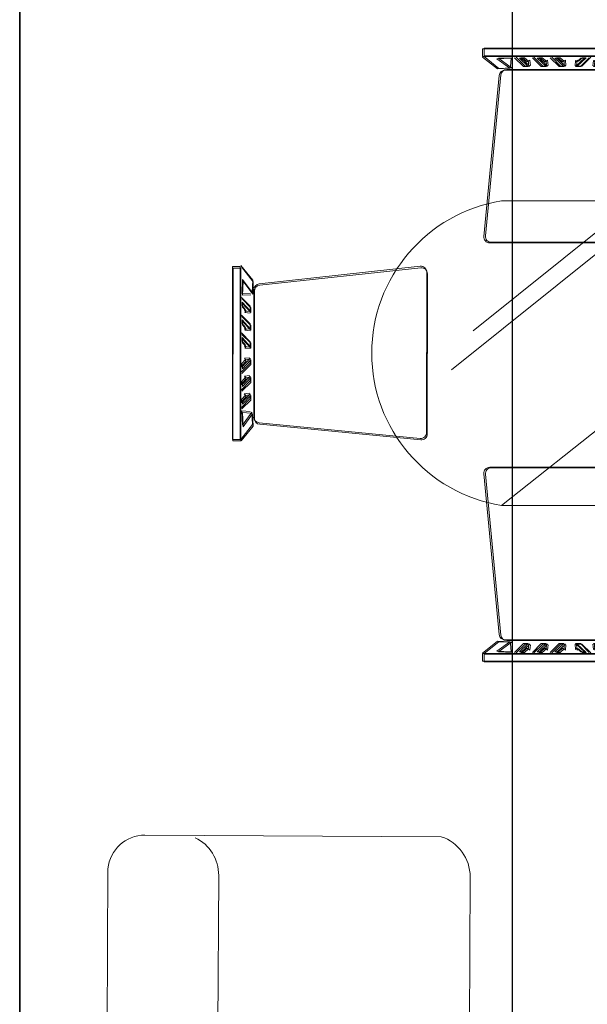
# Model space of a CAD drawing. Units: inches. Extents: x -26 to 575, y -18 to 513.
# Tile 19 of 28: x 278 to 316, y 241 to 307. Entities that reach past the tile are written whole.
import ezdxf

# ---------------------------------------------------------------- set-up
doc = ezdxf.new("R2010")
doc.units = ezdxf.units.IN
doc.header["$MEASUREMENT"] = 0
for name, color, linetype, lineweight in [('A-ANNO-DIMS', 2, 'Continuous', 18), ('A-WALL', 7, 'Continuous', 35), ('Furniture', 8, 'Continuous', 15)]:
    doc.layers.add(name, color=color, linetype=linetype, lineweight=lineweight)
doc.styles.get("Standard").update_dxf_attribs({"font": 'arial.ttf', "height": 6})
doc.dimstyles.get("Standard").update_dxf_attribs({"dimtxt": 6, "dimasz": 0.18, "dimexe": 0.18, "dimexo": 0.0625, "dimgap": 0.09, "dimtad": 0, "dimtih": 1, "dimtoh": 1, "dimzin": 0, "dimdsep": 46, "dimlunit": 3, "dimtxsty": 'Standard', "dimcen": 0.09, "dimadec": 0, "dimazin": 0, "dimtfac": 1, "dimtofl": 0, "dimtmove": 0, "dimatfit": 3, "dimfxl": 1, "dimtolj": 1, "dimtzin": 0, "dimarcsym": 0})

# ---------------------------------------------------------------- blocks, each defined once
blk = doc.blocks.new('DINING-SET-6-SEAT')
for p, q in [((16.828, 40.76, -3.573), (16.828, 41.278, -3.573)), ((16.828, 41.278, -3.573), (28.461, 41.278, -3.573)), ((16.931, 40.798, -3.573), (16.931, 41.316, -3.573)), ((16.931, 41.316, -3.573), (28.564, 41.316, -3.573)), ((28.461, 41.278, -3.573), (28.461, 40.76, -3.573)), ((28.564, 41.316, -3.573), (28.564, 40.798, -3.573)), ((47.187, 41.329, -3.573), (35.554, 41.319, -3.573)), ((35.554, 41.319, -3.573), (35.554, 40.801, -3.573)), ((47.29, 41.291, -3.573), (35.657, 41.281, -3.573)), ((35.657, 41.281, -3.573), (35.657, 40.763, -3.573)), ((47.188, 40.811, -3.573), (47.187, 41.329, -3.573)), ((47.29, 40.774, -3.573), (47.29, 41.291, -3.573)), ((28.461, 40.76, -3.573), (16.828, 40.76, -3.573)), ((16.828, 40.72, -3.573), (17.824, 39.924, -3.573)), ((28.564, 40.798, -3.573), (16.931, 40.798, -3.573)), ((16.931, 40.758, -3.573), (17.927, 39.962, -3.573)), ((17.784, 40.601, -3.573), (18.74, 40.641, -3.573)), ((18.661, 39.964, -3.573), (17.784, 40.601, -3.573)), ((17.887, 40.639, -3.573), (18.843, 40.679, -3.573)), ((18.763, 40.002, -3.573), (17.887, 40.639, -3.573)), ((18.74, 40.641, -3.573), (18.7, 40.083, -3.573)), ((18.843, 40.679, -3.573), (18.803, 40.121, -3.573)), ((18.979, 40.681, -3.573), (19.577, 40.083, -3.573)), ((19.082, 40.718, -3.573), (19.68, 40.121, -3.573)), ((19.896, 40.083, -3.573), (19.298, 40.641, -3.573)), ((19.298, 40.641, -3.573), (19.537, 40.641, -3.573)), ((19.998, 40.121, -3.573), (19.401, 40.679, -3.573)), ((19.401, 40.679, -3.573), (19.64, 40.679, -3.573)), ((19.537, 40.641, -3.573), (19.816, 40.402, -3.573)), ((19.64, 40.679, -3.573), (19.919, 40.44, -3.573)), ((19.816, 40.402, -3.573), (19.896, 40.481, -3.573)), ((19.896, 40.481, -3.573), (19.936, 40.123, -3.573)), ((19.919, 40.44, -3.573), (19.998, 40.519, -3.573)), ((19.998, 40.519, -3.573), (20.038, 40.161, -3.573)), ((20.175, 40.681, -3.573), (20.772, 40.083, -3.573)), ((20.277, 40.718, -3.573), (20.875, 40.121, -3.573)), ((21.091, 40.083, -3.573), (20.493, 40.641, -3.573)), ((20.493, 40.641, -3.573), (20.732, 40.641, -3.573)), ((21.194, 40.121, -3.573), (20.596, 40.679, -3.573)), ((20.596, 40.679, -3.573), (20.835, 40.679, -3.573)), ((20.732, 40.641, -3.573), (21.011, 40.402, -3.573)), ((20.835, 40.679, -3.573), (21.114, 40.44, -3.573)), ((21.011, 40.402, -3.573), (21.091, 40.481, -3.573)), ((21.091, 40.481, -3.573), (21.131, 40.123, -3.573)), ((21.114, 40.44, -3.573), (21.194, 40.519, -3.573)), ((21.194, 40.519, -3.573), (21.233, 40.161, -3.573)), ((21.37, 40.681, -3.573), (21.967, 40.083, -3.573)), ((21.473, 40.718, -3.573), (22.07, 40.121, -3.573)), ((22.286, 40.083, -3.573), (21.688, 40.641, -3.573)), ((21.688, 40.641, -3.573), (21.928, 40.641, -3.573)), ((22.389, 40.121, -3.573), (21.791, 40.679, -3.573)), ((21.791, 40.679, -3.573), (22.03, 40.679, -3.573)), ((21.928, 40.641, -3.573), (22.206, 40.402, -3.573)), ((22.03, 40.679, -3.573), (22.309, 40.44, -3.573)), ((22.206, 40.402, -3.573), (22.286, 40.481, -3.573)), ((22.286, 40.481, -3.573), (22.326, 40.123, -3.573)), ((22.309, 40.44, -3.573), (22.389, 40.519, -3.573)), ((22.389, 40.519, -3.573), (22.429, 40.161, -3.573)), ((23.083, 40.481, -3.573), (23.043, 40.123, -3.573)), ((23.083, 40.083, -3.573), (23.681, 40.641, -3.573)), ((23.163, 40.402, -3.573), (23.083, 40.481, -3.573)), ((23.186, 40.519, -3.573), (23.146, 40.161, -3.573)), ((23.441, 40.641, -3.573), (23.163, 40.402, -3.573)), ((23.186, 40.121, -3.573), (23.783, 40.679, -3.573)), ((23.265, 40.44, -3.573), (23.186, 40.519, -3.573)), ((23.544, 40.679, -3.573), (23.265, 40.44, -3.573)), ((23.999, 40.681, -3.573), (23.402, 40.083, -3.573)), ((23.681, 40.641, -3.573), (23.441, 40.641, -3.573)), ((24.102, 40.718, -3.573), (23.504, 40.121, -3.573)), ((23.783, 40.679, -3.573), (23.544, 40.679, -3.573)), ((24.278, 40.481, -3.573), (24.238, 40.123, -3.573)), ((24.278, 40.083, -3.573), (24.876, 40.641, -3.573)), ((24.358, 40.402, -3.573), (24.278, 40.481, -3.573)), ((24.381, 40.519, -3.573), (24.341, 40.161, -3.573)), ((24.637, 40.641, -3.573), (24.358, 40.402, -3.573)), ((24.381, 40.121, -3.573), (24.978, 40.679, -3.573)), ((24.461, 40.44, -3.573), (24.381, 40.519, -3.573)), ((24.739, 40.679, -3.573), (24.461, 40.44, -3.573)), ((25.194, 40.681, -3.573), (24.597, 40.083, -3.573)), ((24.876, 40.641, -3.573), (24.637, 40.641, -3.573)), ((25.297, 40.718, -3.573), (24.7, 40.121, -3.573)), ((24.978, 40.679, -3.573), (24.739, 40.679, -3.573)), ((25.473, 40.481, -3.573), (25.434, 40.123, -3.573)), ((25.473, 40.083, -3.573), (26.071, 40.641, -3.573)), ((25.553, 40.402, -3.573), (25.473, 40.481, -3.573)), ((25.576, 40.519, -3.573), (25.536, 40.161, -3.573)), ((25.832, 40.641, -3.573), (25.553, 40.402, -3.573)), ((25.576, 40.121, -3.573), (26.174, 40.679, -3.573)), ((25.656, 40.44, -3.573), (25.576, 40.519, -3.573)), ((25.935, 40.679, -3.573), (25.656, 40.44, -3.573)), ((26.39, 40.681, -3.573), (25.792, 40.083, -3.573)), ((26.071, 40.641, -3.573), (25.832, 40.641, -3.573)), ((26.492, 40.718, -3.573), (25.895, 40.121, -3.573)), ((26.174, 40.679, -3.573), (25.935, 40.679, -3.573)), ((27.585, 40.601, -3.573), (26.629, 40.641, -3.573)), ((26.629, 40.641, -3.573), (26.669, 40.083, -3.573)), ((26.708, 39.964, -3.573), (27.585, 40.601, -3.573)), ((27.688, 40.639, -3.573), (26.731, 40.679, -3.573)), ((26.731, 40.679, -3.573), (26.771, 40.121, -3.573)), ((26.811, 40.002, -3.573), (27.688, 40.639, -3.573)), ((28.541, 40.72, -3.573), (27.545, 39.924, -3.573)), ((28.644, 40.758, -3.573), (27.648, 39.962, -3.573)), ((35.475, 40.761, -3.573), (36.471, 39.966, -3.573)), ((35.554, 40.801, -3.573), (47.188, 40.811, -3.573)), ((35.577, 40.723, -3.573), (36.574, 39.928, -3.573)), ((35.657, 40.763, -3.573), (47.29, 40.774, -3.573)), ((36.431, 40.643, -3.573), (37.387, 40.683, -3.573)), ((37.308, 40.006, -3.573), (36.431, 40.643, -3.573)), ((36.534, 40.605, -3.573), (37.49, 40.646, -3.573)), ((37.411, 39.968, -3.573), (36.534, 40.605, -3.573)), ((37.387, 40.683, -3.573), (37.348, 40.126, -3.573)), ((37.49, 40.646, -3.573), (37.45, 40.088, -3.573)), ((37.626, 40.723, -3.573), (38.224, 40.127, -3.573)), ((37.729, 40.686, -3.573), (38.327, 40.089, -3.573)), ((38.543, 40.127, -3.573), (37.945, 40.684, -3.573)), ((37.945, 40.684, -3.573), (38.184, 40.684, -3.573)), ((38.646, 40.089, -3.573), (38.048, 40.646, -3.573)), ((38.048, 40.646, -3.573), (38.287, 40.646, -3.573)), ((38.184, 40.684, -3.573), (38.463, 40.445, -3.573)), ((38.287, 40.646, -3.573), (38.566, 40.408, -3.573)), ((38.463, 40.445, -3.573), (38.543, 40.525, -3.573)), ((38.543, 40.525, -3.573), (38.583, 40.167, -3.573)), ((38.566, 40.408, -3.573), (38.645, 40.487, -3.573)), ((38.645, 40.487, -3.573), (38.685, 40.129, -3.573)), ((38.821, 40.724, -3.573), (39.419, 40.128, -3.573)), ((38.924, 40.687, -3.573), (39.522, 40.09, -3.573)), ((39.738, 40.128, -3.573), (39.14, 40.685, -3.573)), ((39.14, 40.685, -3.573), (39.379, 40.685, -3.573)), ((39.841, 40.09, -3.573), (39.243, 40.647, -3.573)), ((39.243, 40.647, -3.573), (39.482, 40.647, -3.573)), ((39.379, 40.685, -3.573), (39.658, 40.446, -3.573)), ((39.482, 40.647, -3.573), (39.761, 40.409, -3.573)), ((39.658, 40.446, -3.573), (39.738, 40.526, -3.573)), ((39.738, 40.526, -3.573), (39.778, 40.168, -3.573)), ((39.761, 40.409, -3.573), (39.841, 40.488, -3.573)), ((39.841, 40.488, -3.573), (39.881, 40.13, -3.573)), ((40.016, 40.725, -3.573), (40.615, 40.129, -3.573)), ((40.119, 40.688, -3.573), (40.717, 40.091, -3.573)), ((40.933, 40.129, -3.573), (40.335, 40.686, -3.573)), ((40.335, 40.686, -3.573), (40.574, 40.686, -3.573)), ((41.036, 40.091, -3.573), (40.438, 40.648, -3.573)), ((40.438, 40.648, -3.573), (40.677, 40.648, -3.573)), ((40.574, 40.686, -3.573), (40.853, 40.447, -3.573)), ((40.677, 40.648, -3.573), (40.956, 40.41, -3.573)), ((40.853, 40.447, -3.573), (40.933, 40.527, -3.573)), ((40.933, 40.527, -3.573), (40.973, 40.169, -3.573)), ((40.956, 40.41, -3.573), (41.036, 40.489, -3.573)), ((41.036, 40.489, -3.573), (41.076, 40.131, -3.573)), ((41.73, 40.528, -3.573), (41.69, 40.169, -3.573)), ((41.73, 40.13, -3.573), (42.327, 40.688, -3.573)), ((41.81, 40.448, -3.573), (41.73, 40.528, -3.573)), ((41.833, 40.49, -3.573), (41.793, 40.132, -3.573)), ((42.088, 40.687, -3.573), (41.81, 40.448, -3.573)), ((41.833, 40.092, -3.573), (42.43, 40.65, -3.573)), ((41.912, 40.41, -3.573), (41.833, 40.49, -3.573)), ((42.191, 40.65, -3.573), (41.912, 40.41, -3.573)), ((42.646, 40.728, -3.573), (42.049, 40.13, -3.573)), ((42.327, 40.688, -3.573), (42.088, 40.687, -3.573)), ((42.749, 40.69, -3.573), (42.152, 40.092, -3.573)), ((42.43, 40.65, -3.573), (42.191, 40.65, -3.573)), ((42.925, 40.529, -3.573), (42.885, 40.17, -3.573)), ((42.925, 40.131, -3.573), (43.522, 40.689, -3.573)), ((43.005, 40.449, -3.573), (42.925, 40.529, -3.573)), ((43.028, 40.491, -3.573), (42.988, 40.133, -3.573)), ((43.283, 40.688, -3.573), (43.005, 40.449, -3.573)), ((43.028, 40.093, -3.573), (43.625, 40.651, -3.573)), ((43.108, 40.412, -3.573), (43.028, 40.491, -3.573)), ((43.386, 40.651, -3.573), (43.108, 40.412, -3.573)), ((43.841, 40.729, -3.573), (43.244, 40.131, -3.573)), ((43.522, 40.689, -3.573), (43.283, 40.688, -3.573)), ((43.944, 40.691, -3.573), (43.347, 40.093, -3.573)), ((43.625, 40.651, -3.573), (43.386, 40.651, -3.573)), ((44.12, 40.53, -3.573), (44.081, 40.171, -3.573)), ((44.2, 40.45, -3.573), (44.12, 40.53, -3.573)), ((44.121, 40.132, -3.573), (44.718, 40.69, -3.573)), ((44.223, 40.492, -3.573), (44.183, 40.134, -3.573)), ((44.479, 40.69, -3.573), (44.2, 40.45, -3.573)), ((44.223, 40.094, -3.573), (44.82, 40.652, -3.573)), ((44.303, 40.413, -3.573), (44.223, 40.492, -3.573)), ((44.581, 40.652, -3.573), (44.303, 40.413, -3.573)), ((45.036, 40.73, -3.573), (44.439, 40.132, -3.573)), ((44.718, 40.69, -3.573), (44.479, 40.69, -3.573)), ((45.139, 40.692, -3.573), (44.542, 40.094, -3.573)), ((44.82, 40.652, -3.573), (44.581, 40.652, -3.573)), ((46.232, 40.651, -3.573), (45.275, 40.69, -3.573)), ((45.275, 40.69, -3.573), (45.316, 40.133, -3.573)), ((45.356, 40.013, -3.573), (46.232, 40.651, -3.573)), ((46.334, 40.613, -3.573), (45.378, 40.652, -3.573)), ((45.378, 40.652, -3.573), (45.419, 40.095, -3.573)), ((45.458, 39.976, -3.573), (46.334, 40.613, -3.573)), ((47.188, 40.772, -3.573), (46.192, 39.974, -3.573)), ((47.29, 40.734, -3.573), (46.295, 39.936, -3.573)), ((17.824, 39.924, -3.573), (18.661, 39.964, -3.573)), ((17.927, 39.962, -3.573), (18.763, 40.002, -3.573)), ((26.909, 39.844, -3.573), (18.345, 39.844, -3.573)), ((27.012, 39.882, -3.573), (18.448, 39.882, -3.573)), ((19.577, 40.083, -3.573), (19.896, 40.083, -3.573)), ((19.68, 40.121, -3.573), (19.998, 40.121, -3.573)), ((20.772, 40.083, -3.573), (21.091, 40.083, -3.573)), ((20.875, 40.121, -3.573), (21.194, 40.121, -3.573)), ((21.967, 40.083, -3.573), (22.286, 40.083, -3.573)), ((22.07, 40.121, -3.573), (22.389, 40.121, -3.573)), ((23.402, 40.083, -3.573), (23.083, 40.083, -3.573)), ((23.504, 40.121, -3.573), (23.186, 40.121, -3.573)), ((24.597, 40.083, -3.573), (24.278, 40.083, -3.573)), ((24.7, 40.121, -3.573), (24.381, 40.121, -3.573)), ((25.792, 40.083, -3.573), (25.473, 40.083, -3.573)), ((25.895, 40.121, -3.573), (25.576, 40.121, -3.573)), ((27.545, 39.924, -3.573), (26.708, 39.964, -3.573)), ((27.648, 39.962, -3.573), (26.811, 40.002, -3.573)), ((36.471, 39.966, -3.573), (37.308, 40.006, -3.573)), ((36.574, 39.928, -3.573), (37.411, 39.968, -3.573)), ((37.107, 39.887, -3.573), (45.671, 39.894, -3.573)), ((37.21, 39.849, -3.573), (45.774, 39.856, -3.573)), ((38.224, 40.127, -3.573), (38.543, 40.127, -3.573)), ((38.327, 40.089, -3.573), (38.646, 40.089, -3.573)), ((39.419, 40.128, -3.573), (39.738, 40.128, -3.573)), ((39.522, 40.09, -3.573), (39.841, 40.09, -3.573)), ((40.615, 40.129, -3.573), (40.933, 40.129, -3.573)), ((40.717, 40.091, -3.573), (41.036, 40.091, -3.573)), ((42.049, 40.13, -3.573), (41.73, 40.13, -3.573)), ((42.152, 40.092, -3.573), (41.833, 40.092, -3.573)), ((43.244, 40.131, -3.573), (42.925, 40.131, -3.573)), ((43.347, 40.093, -3.573), (43.028, 40.093, -3.573)), ((44.439, 40.132, -3.573), (44.121, 40.132, -3.573)), ((44.542, 40.094, -3.573), (44.223, 40.094, -3.573)), ((46.192, 39.974, -3.573), (45.356, 40.013, -3.573)), ((46.295, 39.936, -3.573), (45.458, 39.976, -3.573)), ((17.949, 39.484, -3.573), (16.91, 28.653, -3.573)), ((18.052, 39.522, -3.573), (17.012, 28.691, -3.573)), ((28.493, 28.659, -3.573), (27.305, 39.489, -3.573)), ((28.595, 28.696, -3.573), (27.408, 39.527, -3.573)), ((35.534, 28.7, -3.573), (36.712, 39.531, -3.573)), ((35.636, 28.662, -3.573), (36.814, 39.494, -3.573)), ((46.068, 39.534, -3.573), (47.117, 28.704, -3.573)), ((46.171, 39.496, -3.573), (47.219, 28.667, -3.573)), ((16.194, 22.294, -1.308), (26.662, 30.717, -1.308)), ((46.474, 31.041, -1.308), (18.1, 31.041, -1.308)), ((14.74, 19.68, -1.308), (28.116, 30.426, -1.308)), ((25.79, 15.904, -1.308), (43.819, 30.136, -1.308)), ((17.306, 28.217, -3.573), (28.097, 28.217, -3.573)), ((17.409, 28.255, -3.573), (28.199, 28.255, -3.573)), ((46.72, 28.268, -3.573), (35.93, 28.258, -3.573)), ((46.823, 28.23, -3.573), (36.033, 28.22, -3.573)), ((18.1, 10.54, -1.308), (39.457, 27.522, -1.308)), ((0, 14.987, -3.573), (0.01, 26.621, -3.573)), ((0.01, 26.621, -3.573), (0.528, 26.62, -3.573)), ((0.037, 14.884, -3.573), (0.048, 26.518, -3.573)), ((0.048, 26.518, -3.573), (0.565, 26.517, -3.573)), ((0.528, 26.62, -3.573), (0.517, 14.987, -3.573)), ((0.565, 26.517, -3.573), (0.555, 14.884, -3.573)), ((0.567, 26.7, -3.573), (1.363, 25.703, -3.573)), ((0.605, 26.597, -3.573), (1.401, 25.6, -3.573)), ((12.629, 26.641, -3.573), (1.797, 25.463, -3.573)), ((12.667, 26.538, -3.573), (1.835, 25.36, -3.573)), ((52.057, 26.538, -3.573), (62.889, 25.36, -3.573)), ((52.095, 26.641, -3.573), (62.926, 25.463, -3.573)), ((64.119, 26.597, -3.573), (63.323, 25.6, -3.573)), ((64.156, 26.7, -3.573), (63.361, 25.703, -3.573)), ((64.676, 26.518, -3.573), (64.159, 26.517, -3.573)), ((64.159, 26.517, -3.573), (64.169, 14.884, -3.573)), ((64.714, 26.621, -3.573), (64.196, 26.62, -3.573)), ((64.196, 26.62, -3.573), (64.207, 14.987, -3.573)), ((64.686, 14.884, -3.573), (64.676, 26.518, -3.573)), ((64.724, 14.987, -3.573), (64.714, 26.621, -3.573)), ((13.061, 15.454, -3.573), (13.071, 26.244, -3.573)), ((13.099, 15.351, -3.573), (13.108, 26.142, -3.573)), ((51.625, 15.351, -3.573), (51.615, 26.142, -3.573)), ((51.663, 15.454, -3.573), (51.653, 26.244, -3.573)), ((0.686, 25.744, -3.573), (0.645, 24.787, -3.573)), ((0.724, 25.641, -3.573), (0.683, 24.685, -3.573)), ((1.322, 24.866, -3.573), (0.686, 25.744, -3.573)), ((1.36, 24.764, -3.573), (0.724, 25.641, -3.573)), ((1.363, 25.703, -3.573), (1.322, 24.866, -3.573)), ((1.401, 25.6, -3.573), (1.36, 24.764, -3.573)), ((63.323, 25.6, -3.573), (63.364, 24.764, -3.573)), ((63.361, 25.703, -3.573), (63.401, 24.866, -3.573)), ((63.364, 24.764, -3.573), (64, 25.641, -3.573)), ((63.401, 24.866, -3.573), (64.038, 25.744, -3.573)), ((64, 25.641, -3.573), (64.041, 24.685, -3.573)), ((64.038, 25.744, -3.573), (64.078, 24.787, -3.573)), ((0.605, 24.548, -3.573), (1.202, 23.95, -3.573)), ((0.645, 24.787, -3.573), (1.203, 24.827, -3.573)), ((0.683, 24.685, -3.573), (1.241, 24.724, -3.573)), ((1.442, 25.067, -3.573), (1.435, 16.503, -3.573)), ((1.48, 24.964, -3.573), (1.472, 16.401, -3.573)), ((63.244, 24.964, -3.573), (63.252, 16.401, -3.573)), ((63.282, 25.067, -3.573), (63.289, 16.503, -3.573)), ((64.041, 24.685, -3.573), (63.483, 24.724, -3.573)), ((64.078, 24.787, -3.573), (63.521, 24.827, -3.573)), ((64.118, 24.548, -3.573), (63.522, 23.95, -3.573)), ((0.643, 24.446, -3.573), (1.24, 23.847, -3.573)), ((1.202, 23.632, -3.573), (0.645, 24.23, -3.573)), ((0.645, 24.23, -3.573), (0.645, 23.991, -3.573)), ((0.645, 23.991, -3.573), (0.883, 23.712, -3.573)), ((0.683, 24.127, -3.573), (0.682, 23.888, -3.573)), ((0.682, 23.888, -3.573), (0.921, 23.609, -3.573)), ((1.24, 23.529, -3.573), (0.683, 24.127, -3.573)), ((1.202, 23.95, -3.573), (1.202, 23.632, -3.573)), ((40.039, 15.033, -1.308), (51.38, 24.327, -1.308)), ((64.081, 24.446, -3.573), (63.484, 23.847, -3.573)), ((63.484, 23.529, -3.573), (64.041, 24.127, -3.573)), ((63.522, 23.632, -3.573), (64.079, 24.23, -3.573)), ((63.522, 23.95, -3.573), (63.522, 23.632, -3.573)), ((64.041, 23.888, -3.573), (63.803, 23.609, -3.573)), ((64.079, 23.991, -3.573), (63.84, 23.712, -3.573)), ((64.041, 24.127, -3.573), (64.041, 23.888, -3.573)), ((64.079, 24.23, -3.573), (64.079, 23.991, -3.573)), ((0.604, 23.353, -3.573), (1.201, 22.755, -3.573)), ((0.642, 23.25, -3.573), (1.239, 22.652, -3.573)), ((0.883, 23.712, -3.573), (0.804, 23.632, -3.573)), ((0.804, 23.632, -3.573), (1.162, 23.592, -3.573)), ((0.921, 23.609, -3.573), (0.841, 23.529, -3.573)), ((0.841, 23.529, -3.573), (1.2, 23.489, -3.573)), ((1.24, 23.847, -3.573), (1.24, 23.529, -3.573)), ((63.484, 23.847, -3.573), (63.484, 23.529, -3.573)), ((64.082, 23.25, -3.573), (63.485, 22.652, -3.573)), ((64.12, 23.353, -3.573), (63.523, 22.755, -3.573)), ((63.882, 23.529, -3.573), (63.524, 23.489, -3.573)), ((63.92, 23.632, -3.573), (63.562, 23.592, -3.573)), ((63.803, 23.609, -3.573), (63.882, 23.529, -3.573)), ((63.84, 23.712, -3.573), (63.92, 23.632, -3.573)), ((1.201, 22.436, -3.573), (0.644, 23.034, -3.573)), ((0.644, 23.034, -3.573), (0.644, 22.795, -3.573)), ((0.644, 22.795, -3.573), (0.882, 22.516, -3.573)), ((0.682, 22.932, -3.573), (0.681, 22.693, -3.573)), ((0.681, 22.693, -3.573), (0.92, 22.414, -3.573)), ((1.239, 22.334, -3.573), (0.682, 22.932, -3.573)), ((1.201, 22.755, -3.573), (1.201, 22.436, -3.573)), ((1.239, 22.652, -3.573), (1.239, 22.334, -3.573)), ((63.485, 22.334, -3.573), (64.042, 22.932, -3.573)), ((63.485, 22.652, -3.573), (63.485, 22.334, -3.573)), ((63.523, 22.436, -3.573), (64.08, 23.034, -3.573)), ((63.523, 22.755, -3.573), (63.523, 22.436, -3.573)), ((64.042, 22.693, -3.573), (63.804, 22.414, -3.573)), ((64.08, 22.795, -3.573), (63.842, 22.516, -3.573)), ((64.042, 22.932, -3.573), (64.042, 22.693, -3.573)), ((64.08, 23.034, -3.573), (64.08, 22.795, -3.573)), ((0.603, 22.158, -3.573), (1.2, 21.56, -3.573)), ((0.641, 22.055, -3.573), (1.238, 21.457, -3.573)), ((0.882, 22.516, -3.573), (0.803, 22.437, -3.573)), ((0.803, 22.437, -3.573), (1.161, 22.397, -3.573)), ((0.92, 22.414, -3.573), (0.84, 22.334, -3.573)), ((0.84, 22.334, -3.573), (1.199, 22.294, -3.573)), ((64.083, 22.055, -3.573), (63.486, 21.457, -3.573)), ((64.121, 22.158, -3.573), (63.524, 21.56, -3.573)), ((63.883, 22.334, -3.573), (63.525, 22.294, -3.573)), ((63.921, 22.437, -3.573), (63.563, 22.397, -3.573)), ((63.804, 22.414, -3.573), (63.883, 22.334, -3.573)), ((63.842, 22.516, -3.573), (63.921, 22.437, -3.573)), ((1.2, 21.241, -3.573), (0.643, 21.839, -3.573)), ((0.643, 21.839, -3.573), (0.643, 21.6, -3.573)), ((0.643, 21.6, -3.573), (0.881, 21.321, -3.573)), ((0.681, 21.736, -3.573), (0.68, 21.497, -3.573)), ((0.68, 21.497, -3.573), (0.919, 21.218, -3.573)), ((1.238, 21.138, -3.573), (0.681, 21.736, -3.573)), ((0.881, 21.321, -3.573), (0.802, 21.241, -3.573)), ((0.802, 21.241, -3.573), (1.16, 21.201, -3.573)), ((0.919, 21.218, -3.573), (0.839, 21.139, -3.573)), ((1.2, 21.56, -3.573), (1.2, 21.241, -3.573)), ((1.238, 21.457, -3.573), (1.238, 21.138, -3.573)), ((63.486, 21.138, -3.573), (64.043, 21.736, -3.573)), ((63.486, 21.457, -3.573), (63.486, 21.138, -3.573)), ((63.524, 21.241, -3.573), (64.081, 21.839, -3.573)), ((63.524, 21.56, -3.573), (63.524, 21.241, -3.573)), ((63.922, 21.241, -3.573), (63.564, 21.201, -3.573)), ((64.043, 21.497, -3.573), (63.805, 21.218, -3.573)), ((63.805, 21.218, -3.573), (63.884, 21.139, -3.573)), ((64.081, 21.6, -3.573), (63.843, 21.321, -3.573)), ((63.843, 21.321, -3.573), (63.922, 21.241, -3.573)), ((64.043, 21.736, -3.573), (64.043, 21.497, -3.573)), ((64.081, 21.839, -3.573), (64.081, 21.6, -3.573)), ((0.839, 21.139, -3.573), (1.198, 21.099, -3.573)), ((63.884, 21.139, -3.573), (63.526, 21.099, -3.573)), ((0.601, 19.529, -3.573), (1.199, 20.126, -3.573)), ((0.639, 19.426, -3.573), (1.237, 20.023, -3.573)), ((1.199, 20.444, -3.573), (0.641, 19.847, -3.573)), ((0.641, 20.086, -3.573), (0.88, 20.365, -3.573)), ((0.641, 19.847, -3.573), (0.641, 20.086, -3.573)), ((1.237, 20.342, -3.573), (0.679, 19.744, -3.573)), ((0.679, 19.983, -3.573), (0.918, 20.262, -3.573)), ((0.679, 19.744, -3.573), (0.679, 19.983, -3.573)), ((0.801, 20.445, -3.573), (1.159, 20.484, -3.573)), ((0.88, 20.365, -3.573), (0.801, 20.445, -3.573)), ((0.839, 20.342, -3.573), (1.197, 20.381, -3.573)), ((0.918, 20.262, -3.573), (0.839, 20.342, -3.573)), ((1.199, 20.126, -3.573), (1.199, 20.444, -3.573)), ((1.237, 20.023, -3.573), (1.237, 20.342, -3.573)), ((34.805, 10.386, -1.308), (47.018, 19.971, -1.308)), ((63.487, 20.023, -3.573), (63.487, 20.342, -3.573)), ((63.487, 20.342, -3.573), (64.045, 19.744, -3.573)), ((64.085, 19.426, -3.573), (63.487, 20.023, -3.573)), ((63.525, 20.126, -3.573), (63.525, 20.444, -3.573)), ((63.525, 20.444, -3.573), (64.083, 19.847, -3.573)), ((64.123, 19.529, -3.573), (63.525, 20.126, -3.573)), ((63.885, 20.342, -3.573), (63.527, 20.381, -3.573)), ((63.923, 20.445, -3.573), (63.565, 20.484, -3.573)), ((63.806, 20.262, -3.573), (63.885, 20.342, -3.573)), ((64.045, 19.983, -3.573), (63.806, 20.262, -3.573)), ((63.843, 20.365, -3.573), (63.923, 20.445, -3.573)), ((64.083, 20.086, -3.573), (63.843, 20.365, -3.573)), ((64.045, 19.744, -3.573), (64.045, 19.983, -3.573)), ((64.083, 19.847, -3.573), (64.083, 20.086, -3.573)), ((1.198, 19.249, -3.573), (0.64, 18.652, -3.573)), ((0.8, 19.249, -3.573), (1.158, 19.289, -3.573)), ((0.879, 19.17, -3.573), (0.8, 19.249, -3.573)), ((1.198, 18.93, -3.573), (1.198, 19.249, -3.573)), ((63.526, 18.93, -3.573), (63.526, 19.249, -3.573)), ((63.526, 19.249, -3.573), (64.084, 18.652, -3.573)), ((63.924, 19.249, -3.573), (63.566, 19.289, -3.573)), ((63.844, 19.17, -3.573), (63.924, 19.249, -3.573)), ((0.6, 18.333, -3.573), (1.198, 18.93, -3.573)), ((0.638, 18.231, -3.573), (1.236, 18.828, -3.573)), ((0.64, 18.891, -3.573), (0.879, 19.17, -3.573)), ((0.64, 18.652, -3.573), (0.64, 18.891, -3.573)), ((1.236, 19.146, -3.573), (0.678, 18.549, -3.573)), ((0.678, 18.788, -3.573), (0.917, 19.067, -3.573)), ((0.678, 18.549, -3.573), (0.678, 18.788, -3.573)), ((0.838, 19.147, -3.573), (1.196, 19.186, -3.573)), ((0.917, 19.067, -3.573), (0.838, 19.147, -3.573)), ((1.236, 18.828, -3.573), (1.236, 19.146, -3.573)), ((63.488, 18.828, -3.573), (63.488, 19.146, -3.573)), ((63.488, 19.146, -3.573), (64.046, 18.549, -3.573)), ((64.086, 18.231, -3.573), (63.488, 18.828, -3.573)), ((64.124, 18.333, -3.573), (63.526, 18.93, -3.573)), ((63.886, 19.147, -3.573), (63.528, 19.186, -3.573)), ((63.807, 19.067, -3.573), (63.886, 19.147, -3.573)), ((64.046, 18.788, -3.573), (63.807, 19.067, -3.573)), ((64.084, 18.891, -3.573), (63.844, 19.17, -3.573)), ((64.046, 18.549, -3.573), (64.046, 18.788, -3.573)), ((64.084, 18.652, -3.573), (64.084, 18.891, -3.573)), ((1.197, 18.054, -3.573), (0.639, 17.457, -3.573)), ((0.639, 17.696, -3.573), (0.878, 17.974, -3.573)), ((1.235, 17.951, -3.573), (0.677, 17.354, -3.573)), ((0.799, 18.054, -3.573), (1.157, 18.094, -3.573)), ((0.878, 17.974, -3.573), (0.799, 18.054, -3.573)), ((0.837, 17.951, -3.573), (1.195, 17.991, -3.573)), ((0.916, 17.872, -3.573), (0.837, 17.951, -3.573)), ((1.197, 17.735, -3.573), (1.197, 18.054, -3.573)), ((1.234, 17.632, -3.573), (1.235, 17.951, -3.573)), ((63.489, 17.632, -3.573), (63.489, 17.951, -3.573)), ((63.489, 17.951, -3.573), (64.047, 17.354, -3.573)), ((63.527, 17.735, -3.573), (63.527, 18.054, -3.573)), ((63.527, 18.054, -3.573), (64.085, 17.457, -3.573)), ((63.887, 17.951, -3.573), (63.529, 17.991, -3.573)), ((63.925, 18.054, -3.573), (63.567, 18.094, -3.573)), ((63.808, 17.872, -3.573), (63.887, 17.951, -3.573)), ((63.846, 17.974, -3.573), (63.925, 18.054, -3.573)), ((64.085, 17.696, -3.573), (63.846, 17.974, -3.573)), ((0.599, 17.138, -3.573), (1.197, 17.735, -3.573)), ((0.637, 17.035, -3.573), (1.234, 17.632, -3.573)), ((0.639, 17.457, -3.573), (0.639, 17.696, -3.573)), ((0.677, 17.593, -3.573), (0.916, 17.872, -3.573)), ((0.677, 17.354, -3.573), (0.677, 17.593, -3.573)), ((64.087, 17.035, -3.573), (63.489, 17.632, -3.573)), ((64.125, 17.138, -3.573), (63.527, 17.735, -3.573)), ((64.047, 17.593, -3.573), (63.808, 17.872, -3.573)), ((64.047, 17.354, -3.573), (64.047, 17.593, -3.573)), ((64.085, 17.457, -3.573), (64.085, 17.696, -3.573)), ((0.677, 15.943, -3.573), (0.639, 16.899, -3.573)), ((0.639, 16.899, -3.573), (1.196, 16.859, -3.573)), ((0.715, 15.84, -3.573), (0.676, 16.796, -3.573)), ((0.676, 16.796, -3.573), (1.234, 16.756, -3.573)), ((1.315, 16.819, -3.573), (0.677, 15.943, -3.573)), ((1.353, 16.716, -3.573), (0.715, 15.84, -3.573)), ((1.354, 15.982, -3.573), (1.315, 16.819, -3.573)), ((1.392, 15.879, -3.573), (1.353, 16.716, -3.573)), ((63.332, 15.879, -3.573), (63.371, 16.716, -3.573)), ((63.369, 15.982, -3.573), (63.408, 16.819, -3.573)), ((63.371, 16.716, -3.573), (64.009, 15.84, -3.573)), ((63.408, 16.819, -3.573), (64.046, 15.943, -3.573)), ((64.048, 16.796, -3.573), (63.49, 16.756, -3.573)), ((64.085, 16.899, -3.573), (63.528, 16.859, -3.573)), ((64.009, 15.84, -3.573), (64.048, 16.796, -3.573)), ((64.046, 15.943, -3.573), (64.085, 16.899, -3.573)), ((0.557, 14.987, -3.573), (1.354, 15.982, -3.573)), ((1.795, 16.106, -3.573), (12.624, 15.058, -3.573)), ((1.832, 16.004, -3.573), (12.662, 14.955, -3.573)), ((62.892, 16.004, -3.573), (52.062, 14.955, -3.573)), ((62.929, 16.106, -3.573), (52.099, 15.058, -3.573)), ((64.167, 14.987, -3.573), (63.369, 15.982, -3.573)), ((0.595, 14.884, -3.573), (1.392, 15.879, -3.573)), ((64.129, 14.884, -3.573), (63.332, 15.879, -3.573)), ((0.517, 14.987, -3.573), (0, 14.987, -3.573)), ((0.555, 14.884, -3.573), (0.037, 14.884, -3.573)), ((64.169, 14.884, -3.573), (64.686, 14.884, -3.573)), ((64.207, 14.987, -3.573), (64.724, 14.987, -3.573)), ((17.949, 1.845, -3.573), (16.91, 12.676, -3.573)), ((18.052, 1.807, -3.573), (17.012, 12.638, -3.573)), ((17.306, 13.113, -3.573), (28.097, 13.113, -3.573)), ((17.409, 13.075, -3.573), (28.199, 13.075, -3.573)), ((28.493, 12.671, -3.573), (27.305, 1.84, -3.573)), ((28.595, 12.633, -3.573), (27.408, 1.802, -3.573)), ((35.534, 12.63, -3.573), (36.712, 1.798, -3.573)), ((35.636, 12.668, -3.573), (36.814, 1.836, -3.573)), ((46.72, 13.062, -3.573), (35.93, 13.071, -3.573)), ((46.823, 13.1, -3.573), (36.033, 13.109, -3.573)), ((46.068, 1.795, -3.573), (47.117, 12.625, -3.573)), ((46.171, 1.833, -3.573), (47.219, 12.663, -3.573)), ((18.1, 10.54, -1.308), (46.474, 10.54, -1.308)), ((16.828, 0.609, -3.573), (17.824, 1.405, -3.573)), ((16.931, 0.571, -3.573), (17.927, 1.367, -3.573)), ((18.661, 1.366, -3.573), (17.784, 0.728, -3.573)), ((17.824, 1.405, -3.573), (18.661, 1.366, -3.573)), ((18.763, 1.328, -3.573), (17.887, 0.691, -3.573)), ((17.927, 1.367, -3.573), (18.763, 1.328, -3.573)), ((26.909, 1.485, -3.573), (18.345, 1.485, -3.573)), ((27.012, 1.447, -3.573), (18.448, 1.447, -3.573)), ((27.545, 1.405, -3.573), (26.708, 1.366, -3.573)), ((26.708, 1.366, -3.573), (27.585, 0.728, -3.573)), ((27.648, 1.367, -3.573), (26.811, 1.328, -3.573)), ((26.811, 1.328, -3.573), (27.688, 0.691, -3.573)), ((28.541, 0.609, -3.573), (27.545, 1.405, -3.573)), ((28.644, 0.571, -3.573), (27.648, 1.367, -3.573)), ((35.475, 0.568, -3.573), (36.471, 1.364, -3.573)), ((35.577, 0.606, -3.573), (36.574, 1.401, -3.573)), ((36.471, 1.364, -3.573), (37.308, 1.323, -3.573)), ((37.411, 1.361, -3.573), (36.534, 0.724, -3.573)), ((36.574, 1.401, -3.573), (37.411, 1.361, -3.573)), ((37.107, 1.443, -3.573), (45.671, 1.435, -3.573)), ((37.21, 1.48, -3.573), (45.774, 1.473, -3.573)), ((46.192, 1.355, -3.573), (45.356, 1.316, -3.573)), ((46.295, 1.393, -3.573), (45.458, 1.354, -3.573)), ((45.458, 1.354, -3.573), (46.334, 0.716, -3.573)), ((47.188, 0.558, -3.573), (46.192, 1.355, -3.573)), ((47.29, 0.596, -3.573), (46.295, 1.393, -3.573)), ((17.784, 0.728, -3.573), (18.74, 0.689, -3.573)), ((17.887, 0.691, -3.573), (18.843, 0.651, -3.573)), ((18.74, 0.689, -3.573), (18.7, 1.246, -3.573)), ((18.843, 0.651, -3.573), (18.803, 1.208, -3.573)), ((18.979, 0.649, -3.573), (19.577, 1.246, -3.573)), ((19.082, 0.611, -3.573), (19.68, 1.208, -3.573)), ((19.896, 1.246, -3.573), (19.298, 0.689, -3.573)), ((19.298, 0.689, -3.573), (19.537, 0.689, -3.573)), ((19.998, 1.208, -3.573), (19.401, 0.651, -3.573)), ((19.537, 0.689, -3.573), (19.816, 0.928, -3.573)), ((19.577, 1.246, -3.573), (19.896, 1.246, -3.573)), ((19.64, 0.651, -3.573), (19.919, 0.89, -3.573)), ((19.68, 1.208, -3.573), (19.998, 1.208, -3.573)), ((19.816, 0.928, -3.573), (19.896, 0.848, -3.573)), ((19.896, 0.848, -3.573), (19.936, 1.206, -3.573)), ((19.919, 0.89, -3.573), (19.998, 0.81, -3.573)), ((19.998, 0.81, -3.573), (20.038, 1.168, -3.573)), ((20.175, 0.649, -3.573), (20.772, 1.246, -3.573)), ((20.277, 0.611, -3.573), (20.875, 1.208, -3.573)), ((21.091, 1.246, -3.573), (20.493, 0.689, -3.573)), ((20.493, 0.689, -3.573), (20.732, 0.689, -3.573)), ((21.194, 1.208, -3.573), (20.596, 0.651, -3.573)), ((20.732, 0.689, -3.573), (21.011, 0.928, -3.573)), ((20.772, 1.246, -3.573), (21.091, 1.246, -3.573)), ((20.835, 0.651, -3.573), (21.114, 0.89, -3.573)), ((20.875, 1.208, -3.573), (21.194, 1.208, -3.573)), ((21.011, 0.928, -3.573), (21.091, 0.848, -3.573)), ((21.091, 0.848, -3.573), (21.131, 1.206, -3.573)), ((21.114, 0.89, -3.573), (21.194, 0.81, -3.573)), ((21.194, 0.81, -3.573), (21.233, 1.168, -3.573)), ((21.37, 0.649, -3.573), (21.967, 1.246, -3.573)), ((21.473, 0.611, -3.573), (22.07, 1.208, -3.573)), ((22.286, 1.246, -3.573), (21.688, 0.689, -3.573)), ((21.688, 0.689, -3.573), (21.928, 0.689, -3.573)), ((22.389, 1.208, -3.573), (21.791, 0.651, -3.573)), ((21.928, 0.689, -3.573), (22.206, 0.928, -3.573)), ((21.967, 1.246, -3.573), (22.286, 1.246, -3.573)), ((22.03, 0.651, -3.573), (22.309, 0.89, -3.573)), ((22.07, 1.208, -3.573), (22.389, 1.208, -3.573)), ((22.206, 0.928, -3.573), (22.286, 0.848, -3.573)), ((22.286, 0.848, -3.573), (22.326, 1.206, -3.573)), ((22.309, 0.89, -3.573), (22.389, 0.81, -3.573)), ((22.389, 0.81, -3.573), (22.429, 1.168, -3.573)), ((23.083, 0.848, -3.573), (23.043, 1.206, -3.573)), ((23.402, 1.246, -3.573), (23.083, 1.246, -3.573)), ((23.083, 1.246, -3.573), (23.681, 0.689, -3.573)), ((23.163, 0.928, -3.573), (23.083, 0.848, -3.573)), ((23.186, 0.81, -3.573), (23.146, 1.168, -3.573)), ((23.441, 0.689, -3.573), (23.163, 0.928, -3.573)), ((23.504, 1.208, -3.573), (23.186, 1.208, -3.573)), ((23.186, 1.208, -3.573), (23.783, 0.651, -3.573)), ((23.265, 0.89, -3.573), (23.186, 0.81, -3.573)), ((23.544, 0.651, -3.573), (23.265, 0.89, -3.573)), ((23.999, 0.649, -3.573), (23.402, 1.246, -3.573)), ((23.681, 0.689, -3.573), (23.441, 0.689, -3.573)), ((24.102, 0.611, -3.573), (23.504, 1.208, -3.573)), ((24.278, 0.848, -3.573), (24.238, 1.206, -3.573)), ((24.597, 1.246, -3.573), (24.278, 1.246, -3.573)), ((24.278, 1.246, -3.573), (24.876, 0.689, -3.573)), ((24.358, 0.928, -3.573), (24.278, 0.848, -3.573)), ((24.381, 0.81, -3.573), (24.341, 1.168, -3.573)), ((24.637, 0.689, -3.573), (24.358, 0.928, -3.573)), ((24.7, 1.208, -3.573), (24.381, 1.208, -3.573)), ((24.381, 1.208, -3.573), (24.978, 0.651, -3.573)), ((24.461, 0.89, -3.573), (24.381, 0.81, -3.573)), ((24.739, 0.651, -3.573), (24.461, 0.89, -3.573)), ((25.194, 0.649, -3.573), (24.597, 1.246, -3.573)), ((24.876, 0.689, -3.573), (24.637, 0.689, -3.573)), ((25.297, 0.611, -3.573), (24.7, 1.208, -3.573)), ((25.473, 0.848, -3.573), (25.434, 1.206, -3.573)), ((25.792, 1.246, -3.573), (25.473, 1.246, -3.573)), ((25.473, 1.246, -3.573), (26.071, 0.689, -3.573)), ((25.553, 0.928, -3.573), (25.473, 0.848, -3.573)), ((25.576, 0.81, -3.573), (25.536, 1.168, -3.573)), ((25.832, 0.689, -3.573), (25.553, 0.928, -3.573)), ((25.895, 1.208, -3.573), (25.576, 1.208, -3.573)), ((25.576, 1.208, -3.573), (26.174, 0.651, -3.573)), ((25.656, 0.89, -3.573), (25.576, 0.81, -3.573)), ((25.935, 0.651, -3.573), (25.656, 0.89, -3.573)), ((26.39, 0.649, -3.573), (25.792, 1.246, -3.573)), ((26.071, 0.689, -3.573), (25.832, 0.689, -3.573)), ((26.492, 0.611, -3.573), (25.895, 1.208, -3.573)), ((26.629, 0.689, -3.573), (26.669, 1.246, -3.573)), ((27.585, 0.728, -3.573), (26.629, 0.689, -3.573)), ((26.731, 0.651, -3.573), (26.771, 1.208, -3.573)), ((27.688, 0.691, -3.573), (26.731, 0.651, -3.573)), ((37.308, 1.323, -3.573), (36.431, 0.687, -3.573)), ((36.431, 0.687, -3.573), (37.387, 0.646, -3.573)), ((36.534, 0.724, -3.573), (37.49, 0.684, -3.573)), ((37.387, 0.646, -3.573), (37.348, 1.204, -3.573)), ((37.49, 0.684, -3.573), (37.45, 1.241, -3.573)), ((37.626, 0.606, -3.573), (38.224, 1.203, -3.573)), ((37.729, 0.644, -3.573), (38.327, 1.241, -3.573)), ((38.543, 1.203, -3.573), (37.945, 0.646, -3.573)), ((38.646, 1.24, -3.573), (38.048, 0.683, -3.573)), ((38.048, 0.683, -3.573), (38.287, 0.683, -3.573)), ((38.184, 0.645, -3.573), (38.463, 0.884, -3.573)), ((38.224, 1.203, -3.573), (38.543, 1.203, -3.573)), ((38.287, 0.683, -3.573), (38.566, 0.922, -3.573)), ((38.327, 1.241, -3.573), (38.646, 1.24, -3.573)), ((38.463, 0.884, -3.573), (38.543, 0.804, -3.573)), ((38.543, 0.804, -3.573), (38.583, 1.163, -3.573)), ((38.566, 0.922, -3.573), (38.645, 0.842, -3.573)), ((38.645, 0.842, -3.573), (38.685, 1.2, -3.573)), ((38.821, 0.605, -3.573), (39.419, 1.202, -3.573)), ((38.924, 0.643, -3.573), (39.522, 1.24, -3.573)), ((39.738, 1.201, -3.573), (39.14, 0.645, -3.573)), ((39.841, 1.239, -3.573), (39.243, 0.682, -3.573)), ((39.243, 0.682, -3.573), (39.482, 0.682, -3.573)), ((39.379, 0.644, -3.573), (39.658, 0.883, -3.573)), ((39.419, 1.202, -3.573), (39.738, 1.201, -3.573)), ((39.482, 0.682, -3.573), (39.761, 0.921, -3.573)), ((39.522, 1.24, -3.573), (39.841, 1.239, -3.573)), ((39.658, 0.883, -3.573), (39.738, 0.803, -3.573)), ((39.738, 0.803, -3.573), (39.778, 1.162, -3.573)), ((39.761, 0.921, -3.573), (39.841, 0.841, -3.573)), ((39.841, 0.841, -3.573), (39.881, 1.199, -3.573)), ((40.016, 0.604, -3.573), (40.615, 1.201, -3.573)), ((40.119, 0.642, -3.573), (40.717, 1.238, -3.573)), ((40.933, 1.2, -3.573), (40.335, 0.643, -3.573)), ((41.036, 1.238, -3.573), (40.438, 0.681, -3.573)), ((40.438, 0.681, -3.573), (40.677, 0.681, -3.573)), ((40.574, 0.643, -3.573), (40.853, 0.882, -3.573)), ((40.615, 1.201, -3.573), (40.933, 1.2, -3.573)), ((40.677, 0.681, -3.573), (40.956, 0.92, -3.573)), ((40.717, 1.238, -3.573), (41.036, 1.238, -3.573)), ((40.853, 0.882, -3.573), (40.933, 0.802, -3.573)), ((40.933, 0.802, -3.573), (40.973, 1.161, -3.573)), ((40.956, 0.92, -3.573), (41.036, 0.84, -3.573)), ((41.036, 0.84, -3.573), (41.076, 1.198, -3.573)), ((41.73, 0.802, -3.573), (41.69, 1.16, -3.573)), ((42.049, 1.199, -3.573), (41.73, 1.2, -3.573)), ((41.73, 1.2, -3.573), (42.327, 0.642, -3.573)), ((41.81, 0.881, -3.573), (41.73, 0.802, -3.573)), ((41.833, 0.839, -3.573), (41.793, 1.198, -3.573)), ((42.088, 0.642, -3.573), (41.81, 0.881, -3.573)), ((42.152, 1.237, -3.573), (41.833, 1.238, -3.573)), ((41.833, 1.238, -3.573), (42.43, 0.679, -3.573)), ((41.912, 0.919, -3.573), (41.833, 0.839, -3.573)), ((42.191, 0.68, -3.573), (41.912, 0.919, -3.573)), ((42.646, 0.602, -3.573), (42.049, 1.199, -3.573)), ((42.749, 0.639, -3.573), (42.152, 1.237, -3.573)), ((42.43, 0.679, -3.573), (42.191, 0.68, -3.573)), ((42.925, 0.8, -3.573), (42.885, 1.159, -3.573)), ((43.244, 1.198, -3.573), (42.925, 1.199, -3.573)), ((42.925, 1.199, -3.573), (43.522, 0.641, -3.573)), ((43.005, 0.88, -3.573), (42.925, 0.8, -3.573)), ((43.028, 0.838, -3.573), (42.988, 1.197, -3.573)), ((43.283, 0.641, -3.573), (43.005, 0.88, -3.573)), ((43.347, 1.236, -3.573), (43.028, 1.236, -3.573)), ((43.028, 1.236, -3.573), (43.625, 0.678, -3.573)), ((43.108, 0.918, -3.573), (43.028, 0.838, -3.573)), ((43.386, 0.679, -3.573), (43.108, 0.918, -3.573)), ((43.841, 0.601, -3.573), (43.244, 1.198, -3.573)), ((43.944, 0.638, -3.573), (43.347, 1.236, -3.573)), ((43.625, 0.678, -3.573), (43.386, 0.679, -3.573)), ((44.12, 0.799, -3.573), (44.081, 1.158, -3.573)), ((44.2, 0.879, -3.573), (44.12, 0.799, -3.573)), ((44.439, 1.197, -3.573), (44.121, 1.198, -3.573)), ((44.121, 1.198, -3.573), (44.718, 0.64, -3.573)), ((44.223, 0.837, -3.573), (44.183, 1.196, -3.573)), ((44.479, 0.64, -3.573), (44.2, 0.879, -3.573)), ((44.542, 1.235, -3.573), (44.223, 1.235, -3.573)), ((44.223, 1.235, -3.573), (44.82, 0.677, -3.573)), ((44.303, 0.917, -3.573), (44.223, 0.837, -3.573)), ((44.581, 0.678, -3.573), (44.303, 0.917, -3.573)), ((45.036, 0.6, -3.573), (44.439, 1.197, -3.573)), ((45.139, 0.637, -3.573), (44.542, 1.235, -3.573)), ((44.82, 0.677, -3.573), (44.581, 0.678, -3.573)), ((45.275, 0.639, -3.573), (45.316, 1.197, -3.573)), ((46.232, 0.678, -3.573), (45.275, 0.639, -3.573)), ((45.356, 1.316, -3.573), (46.232, 0.678, -3.573)), ((45.378, 0.677, -3.573), (45.419, 1.234, -3.573)), ((46.334, 0.716, -3.573), (45.378, 0.677, -3.573)), ((28.461, 0.569, -3.573), (16.828, 0.569, -3.573)), ((16.828, 0.569, -3.573), (16.828, 0.051, -3.573)), ((16.828, 0.051, -3.573), (28.461, 0.051, -3.573)), ((28.564, 0.531, -3.573), (16.931, 0.531, -3.573)), ((16.931, 0.531, -3.573), (16.931, 0.014, -3.573)), ((16.931, 0.014, -3.573), (28.564, 0.014, -3.573)), ((19.401, 0.651, -3.573), (19.64, 0.651, -3.573)), ((20.596, 0.651, -3.573), (20.835, 0.651, -3.573)), ((21.791, 0.651, -3.573), (22.03, 0.651, -3.573)), ((23.783, 0.651, -3.573), (23.544, 0.651, -3.573)), ((24.978, 0.651, -3.573), (24.739, 0.651, -3.573)), ((26.174, 0.651, -3.573), (25.935, 0.651, -3.573)), ((28.461, 0.051, -3.573), (28.461, 0.569, -3.573)), ((28.564, 0.014, -3.573), (28.564, 0.531, -3.573)), ((35.554, 0.011, -3.573), (35.554, 0.528, -3.573)), ((35.554, 0.528, -3.573), (47.188, 0.518, -3.573)), ((47.187, 0, -3.573), (35.554, 0.011, -3.573)), ((35.657, 0.048, -3.573), (35.657, 0.566, -3.573)), ((35.657, 0.566, -3.573), (47.29, 0.556, -3.573)), ((47.29, 0.038, -3.573), (35.657, 0.048, -3.573)), ((37.945, 0.646, -3.573), (38.184, 0.645, -3.573)), ((39.14, 0.645, -3.573), (39.379, 0.644, -3.573)), ((40.335, 0.643, -3.573), (40.574, 0.643, -3.573)), ((42.327, 0.642, -3.573), (42.088, 0.642, -3.573)), ((43.522, 0.641, -3.573), (43.283, 0.641, -3.573)), ((44.718, 0.64, -3.573), (44.479, 0.64, -3.573)), ((47.188, 0.518, -3.573), (47.187, 0, -3.573)), ((47.29, 0.556, -3.573), (47.29, 0.038, -3.573))]:
    blk.add_line(p, q)
for centre, radius, start, end in [((18.345, 39.446, -3.573), 0.398, 90, 174.51988), ((18.448, 39.484, -3.573), 0.398, 90, 174.51988), ((26.909, 39.446, -3.573), 0.398, 6.25717, 90), ((27.012, 39.484, -3.573), 0.398, 6.25717, 90), ((37.108, 39.488, -3.573), 0.398, 90.05022, 173.79305), ((37.211, 39.45, -3.573), 0.398, 90.05022, 173.79305), ((45.671, 39.496, -3.573), 0.398, 5.53034, 90.05022), ((45.774, 39.458, -3.573), 0.398, 5.53034, 90.05022), ((19.748, 20.791, -1.308), 10.382, 99.13208, 260.86792), ((44.826, 20.791, -1.308), 10.382, 279.13208, 80.86792), ((17.306, 28.615, -3.573), 0.398, 174.51988, 270), ((17.409, 28.653, -3.573), 0.398, 174.51988, 270), ((28.097, 28.615, -3.573), 0.398, 270, 6.25717), ((28.199, 28.653, -3.573), 0.398, 270, 6.25717), ((35.93, 28.656, -3.573), 0.398, 173.79305, 270.05022), ((36.032, 28.619, -3.573), 0.398, 173.79305, 270.05022), ((46.72, 28.666, -3.573), 0.398, 270.05022, 5.53034), ((46.823, 28.628, -3.573), 0.398, 270.05022, 5.53034), ((12.672, 26.245, -3.573), 0.398, 359.94978, 96.20695), ((12.71, 26.142, -3.573), 0.398, 359.94978, 96.20695), ((52.014, 26.142, -3.573), 0.398, 83.79305, 180.05022), ((52.052, 26.245, -3.573), 0.398, 83.79305, 180.05022), ((1.84, 25.067, -3.573), 0.398, 96.20695, 179.94978), ((1.878, 24.964, -3.573), 0.398, 96.20695, 179.94978), ((62.846, 24.964, -3.573), 0.398, 0.05022, 83.79305), ((62.883, 25.067, -3.573), 0.398, 0.05022, 83.79305), ((1.833, 16.503, -3.573), 0.398, 179.94978, 264.46966), ((1.871, 16.4, -3.573), 0.398, 179.94978, 264.46966), ((62.853, 16.4, -3.573), 0.398, 275.53034, 0.05022), ((62.891, 16.503, -3.573), 0.398, 275.53034, 0.05022), ((12.663, 15.454, -3.573), 0.398, 264.46966, 359.94978), ((12.701, 15.352, -3.573), 0.398, 264.46966, 359.94978), ((52.023, 15.352, -3.573), 0.398, 180.05022, 275.53034), ((52.061, 15.454, -3.573), 0.398, 180.05022, 275.53034), ((17.306, 12.714, -3.573), 0.398, 90, 185.48012), ((17.409, 12.676, -3.573), 0.398, 90, 185.48012), ((28.097, 12.714, -3.573), 0.398, 353.74283, 90), ((28.199, 12.676, -3.573), 0.398, 353.74283, 90), ((35.93, 12.673, -3.573), 0.398, 89.94978, 186.20695), ((36.032, 12.711, -3.573), 0.398, 89.94978, 186.20695), ((46.72, 12.663, -3.573), 0.398, 354.46966, 89.94978), ((46.823, 12.701, -3.573), 0.398, 354.46966, 89.94978), ((18.345, 1.883, -3.573), 0.398, 185.48012, 270), ((18.448, 1.846, -3.573), 0.398, 185.48012, 270), ((26.909, 1.883, -3.573), 0.398, 270, 353.74283), ((27.012, 1.846, -3.573), 0.398, 270, 353.74283), ((37.108, 1.841, -3.573), 0.398, 186.20695, 269.94978), ((37.211, 1.879, -3.573), 0.398, 186.20695, 269.94978), ((45.671, 1.834, -3.573), 0.398, 269.94978, 354.46966), ((45.774, 1.871, -3.573), 0.398, 269.94978, 354.46966)]:
    blk.add_arc(centre, radius, start, end)
blk = doc.blocks.new('SOFA-L-SECTIONAL')
for p, q in [((22.738, 97.988, -13.498), (2.817, 98.09, -13.498)), ((0.328, 95.831, -13.498), (0.235, 77.862, -13.498)), ((7.684, 77.72, -13.498), (7.775, 95.38, -13.498)), ((24.594, 77.633, -13.498), (24.685, 95.292, -13.498))]:
    blk.add_line(p, q)
for centre, radius, start, end in [((2.804, 95.604, -13.498), 2.487, 89.70451, 174.75427), ((4.956, 95.394, -13.498), 2.819, 359.70451, 63.77883), ((21.867, 95.307, -13.498), 2.819, 359.70451, 71.99328)]:
    blk.add_arc(centre, radius, start, end)
blk = doc.blocks.new('*D26')
at = {"layer": 'A-ANNO-DIMS', "color": 0, "lineweight": -2, "transparency": 16777216}
for p, q in [((337.628, 252.609), (352.461, 252.609)), ((352.281, 252.429), (352.281, 206.753)), ((352.281, 154.689), (352.281, 200.364)), ((337.628, 154.509), (352.461, 154.509))]:
    blk.add_line(p, q, dxfattribs=at)
at = {"layer": 'A-ANNO-DIMS', "color": 0, "transparency": 16777216}
for points in [[(352.251, 252.429), (352.311, 252.429), (352.281, 252.609)], [(352.251, 154.689), (352.311, 154.689), (352.281, 154.509)]]:
    blk.add_solid(points, dxfattribs=at)
at = {"layer": 'Defpoints', "color": 0, "transparency": 16777216}
for p in [(337.566, 252.609), (352.281, 252.609), (337.566, 154.509)]:
    blk.add_point(p, dxfattribs=at)
at = {"layer": 'A-ANNO-DIMS', "color": 0, "transparency": 16777216, "insert": (352.281, 203.559), "char_height": 6, "attachment_point": 5}
blk.add_mtext('\\A1;SECTIONAL SOFA 8\'-2" TYP.', dxfattribs=at)
blk = doc.blocks.new('*D31')
at = {"layer": 'A-ANNO-DIMS', "color": 0, "lineweight": -2, "transparency": 16777216}
for p, q in [((311.292, 466.445), (311.292, -8.972)), ((336.72, 466.445), (336.72, -8.972)), ((311.472, -8.792), (336.54, -8.792)), ((336.72, -8.792), (336.9, -8.792))]:
    blk.add_line(p, q, dxfattribs=at)
at = {"layer": 'A-ANNO-DIMS', "color": 0, "transparency": 16777216}
for points in [[(311.472, -8.762), (311.472, -8.822), (311.292, -8.792)], [(336.54, -8.762), (336.54, -8.822), (336.72, -8.792)]]:
    blk.add_solid(points, dxfattribs=at)
at = {"layer": 'Defpoints', "color": 0, "transparency": 16777216}
for p in [(311.292, 466.508), (336.72, 466.508), (336.72, -8.792)]:
    blk.add_point(p, dxfattribs=at)
at = {"layer": 'A-ANNO-DIMS', "color": 0, "transparency": 16777216, "insert": (352.006, -8.792), "char_height": 6, "attachment_point": 5}
blk.add_mtext('\\A1;2\'-1 1/2"', dxfattribs=at)
blk = doc.blocks.new('*D47')
at = {"layer": 'A-ANNO-DIMS', "color": 0, "lineweight": -2, "transparency": 16777216}
for p, q in [((278.177, 466.445), (278.177, -8.972)), ((311.292, 466.445), (311.292, -8.972)), ((278.357, -8.792), (286.619, -8.792)), ((311.112, -8.792), (302.851, -8.792))]:
    blk.add_line(p, q, dxfattribs=at)
at = {"layer": 'A-ANNO-DIMS', "color": 0, "transparency": 16777216}
for points in [[(278.357, -8.762), (278.357, -8.822), (278.177, -8.792)], [(311.112, -8.762), (311.112, -8.822), (311.292, -8.792)]]:
    blk.add_solid(points, dxfattribs=at)
at = {"layer": 'Defpoints', "color": 0, "transparency": 16777216}
for p in [(278.177, 466.508), (311.292, 466.508), (311.292, -8.792)]:
    blk.add_point(p, dxfattribs=at)
at = {"layer": 'A-ANNO-DIMS', "color": 0, "transparency": 16777216, "insert": (294.735, -8.792), "char_height": 6, "attachment_point": 5}
blk.add_mtext('\\A1;2\'-9"', dxfattribs=at)

msp = doc.modelspace()

# ---------------------------------------------------------------- linework, layer by layer
at = {"layer": 'A-WALL'}
msp.add_line((278.177, 127.508), (278.177, 330.008), dxfattribs=at)

# ---------------------------------------------------------------- block references
at = {"layer": 'Furniture'}
for name, p in [('DINING-SET-6-SEAT', (292.485, 264.256)), ('SOFA-L-SECTIONAL', (283.784, 154.512))]:
    msp.add_blockref(name, p, dxfattribs=at)

# ---------------------------------------------------------------- dimensions: what is measured, and where the dimension line sits
at = {"layer": 'A-ANNO-DIMS'}
for base, p1, p2, picture, middle in [((311.292, -8.792), (278.177, 466.508), (311.292, 466.508), '*D47', (294.735, -8.792)), ((336.72, -8.792), (311.292, 466.508), (336.72, 466.508), '*D31', (352.006, -8.792))]:
    dim = msp.add_linear_dim(base=base, p1=p1, p2=p2, dimstyle='Standard', override={"dimdec": 1, "dimlfac": 1, "dimrnd": 0, "dimzin": 1, "dimdsep": 46, "dimlunit": 4, "dimfrac": 2}, dxfattribs=at)
    dim.commit()
    dim.dimension.update_dxf_attribs({"geometry": picture, "text_midpoint": middle})
dim = msp.add_linear_dim(base=(352.281, 252.609), p1=(337.566, 154.509), p2=(337.566, 252.609), angle=90, text='SECTIONAL SOFA <> TYP.', dimstyle='Standard', override={"dimdec": 1, "dimlfac": 1, "dimrnd": 0, "dimzin": 1, "dimdsep": 46, "dimlunit": 4, "dimfrac": 2}, dxfattribs=at)
dim.commit()
dim.dimension.update_dxf_attribs({"geometry": '*D26', "text_midpoint": (352.281, 203.559)})

doc.saveas('drawing.dxf')
